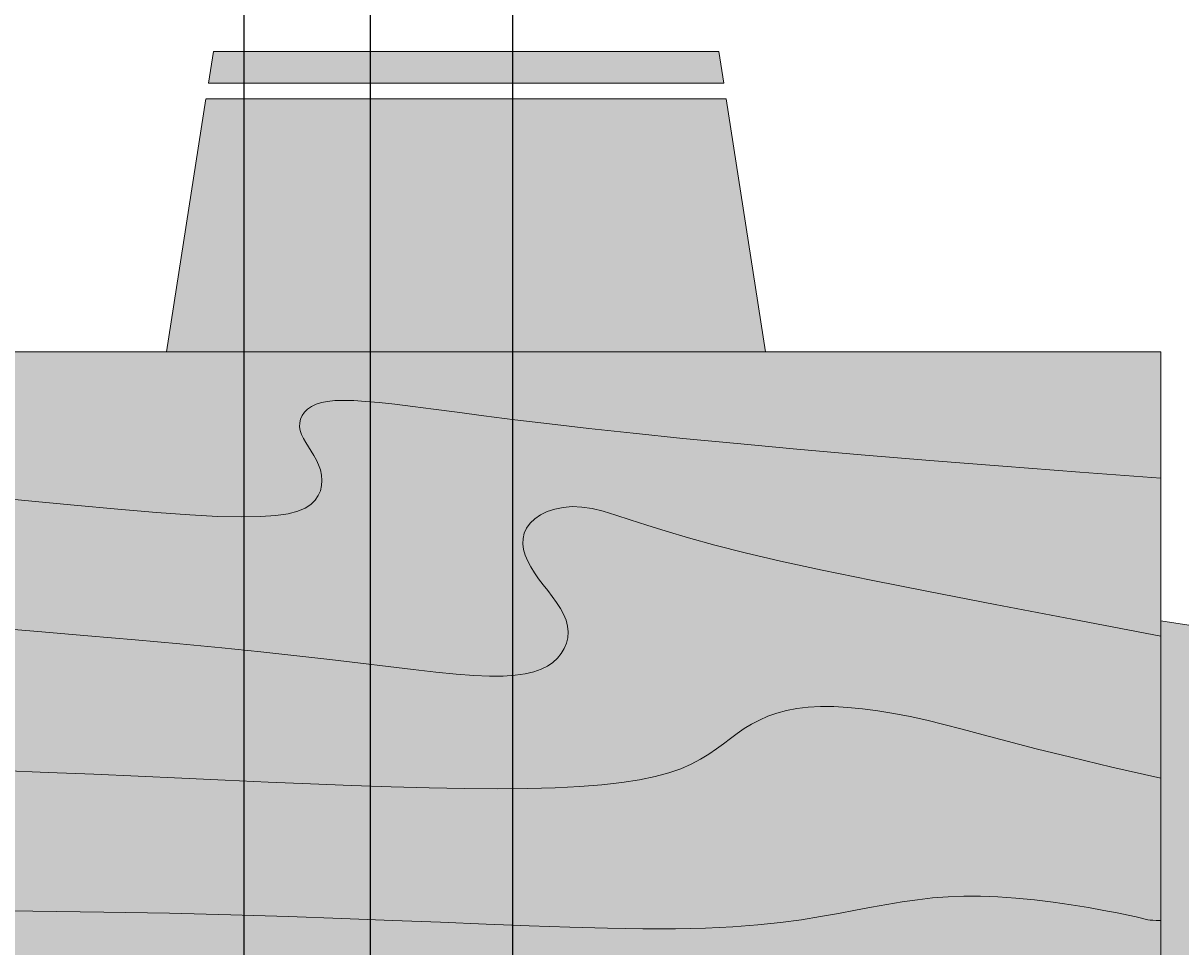
# Model space of a CAD drawing. Units: inches. Extents: x 1567 to 1964, y 1813 to 2447.
# Tile 20 of 28: x 1788 to 1825, y 2199 to 2228. Entities that reach past the tile are written whole.
import ezdxf

# ---------------------------------------------------------------- set-up
doc = ezdxf.new("R2010")
doc.units = ezdxf.units.IN
doc.layers.add('A-ANNO-DIMS', color=2, linetype='Continuous', lineweight=18)
doc.layers.add('A-FURN', color=8, linetype='Continuous', lineweight=18)
doc.layers.add('A-FURN-PATT', color=252, linetype='Continuous', lineweight=13, true_color=0x939598)
doc.styles.get("Standard").update_dxf_attribs({"font": 'arial.ttf'})
doc.dimstyles.get("Standard").update_dxf_attribs({"dimtxt": 0.18, "dimasz": 0.18, "dimexe": 0.18, "dimexo": 0.0625, "dimgap": 0.09, "dimtad": 0, "dimtih": 1, "dimtoh": 1, "dimdec": 4, "dimzin": 0, "dimdsep": 46, "dimtxsty": 'Standard', "dimcen": 0.09, "dimadec": 0, "dimazin": 0, "dimtfac": 1, "dimtdec": 4, "dimtofl": 0, "dimtmove": 0, "dimatfit": 3, "dimfxl": 1, "dimtolj": 1, "dimtzin": 0, "dimarcsym": 0})

# ---------------------------------------------------------------- blocks, each defined once
blk = doc.blocks.new('Dining Set - 36 x 72 in.')
for p, q in [((6, 27.5), (5.8438, 26.50042)), ((6, 27.5), (22, 27.5)), ((22.1563, 26.49966), (22, 27.5)), ((22.1584, 26.5), (5.8466, 26.5)), ((5.7657, 26.00059), (4.5153, 17.99762)), ((5.7696, 26), (22.2392, 26)), ((23.4848, 17.99762), (22.2345, 25.99926)), ((36, 18), (-36, 18)), ((36, -18), (36, 18)), ((44.0006, 8.23428), (35.9976, 9.48474))]:
    blk.add_line(p, q)
for points in [[(-1.6954, 13.45508), (0.0365, 13.29166), (1.5945, 13.14388), (2.9811, 13.01562), (4.1988, 12.9108), (5.25, 12.83333), (6.1393, 12.78613), (6.8802, 12.76823), (7.4883, 12.77767), (7.9792, 12.8125), (8.3685, 12.87077), (8.6719, 12.95052), (8.9049, 13.0498), (9.0833, 13.16666), (9.2205, 13.29899), (9.3216, 13.44401), (9.3895, 13.59879), (9.4271, 13.76041), (9.4373, 13.92594), (9.4232, 14.09245), (9.3875, 14.257), (9.3333, 14.41666), (9.2638, 14.56917), (9.1836, 14.71484), (9.0975, 14.85465), (9.0104, 14.98958), (8.9272, 15.1206), (8.8529, 15.2487), (8.7922, 15.37483), (8.75, 15.5), (8.7305, 15.62467), (8.7344, 15.74739), (8.7617, 15.86621), (8.8125, 15.97916), (8.8867, 16.08431), (8.9844, 16.17968), (9.1055, 16.26334), (9.25, 16.33333), (9.4189, 16.38802), (9.6172, 16.42708), (9.8506, 16.45052), (10.125, 16.45833), (10.4463, 16.45052), (10.8203, 16.42708), (11.2529, 16.38802), (11.75, 16.33333), (12.3184, 16.26318), (12.9694, 16.17838), (13.7151, 16.07991), (14.5677, 15.96875), (15.5395, 15.84586), (16.6426, 15.71224), (17.8893, 15.56884), (19.2917, 15.41666), (20.859, 15.25667), (22.5879, 15.08984), (24.4721, 14.91715), (26.5052, 14.73958), (28.6809, 14.5581), (30.9929, 14.3737), (33.4347, 14.18733), (36, 14)], [(-1.2246, 9.28515), (0.4415, 9.14534), (2.026, 9.01041), (3.5266, 8.87939), (4.9408, 8.7513), (6.266, 8.62516), (7.5, 8.5), (8.6411, 8.37549), (9.6914, 8.2539), (10.6538, 8.13818), (11.5312, 8.03125), (12.3267, 7.93603), (13.043, 7.85547), (13.6831, 7.79248), (14.25, 7.75), (14.7471, 7.7303), (15.1797, 7.73307), (15.5537, 7.75732), (15.875, 7.80208), (16.1494, 7.86637), (16.3828, 7.94922), (16.5811, 8.04964), (16.75, 8.16666), (16.8944, 8.29915), (17.0143, 8.44531), (17.1089, 8.60319), (17.1771, 8.77083), (17.218, 8.94629), (17.2305, 9.1276), (17.2137, 9.31282), (17.1667, 9.5), (17.0895, 9.6875), (16.987, 9.875), (16.8649, 10.0625), (16.7292, 10.25), (16.5856, 10.4375), (16.4401, 10.625), (16.2985, 10.8125), (16.1667, 11), (16.05, 11.18733), (15.9518, 11.3737), (15.8752, 11.5581), (15.8229, 11.73958), (15.798, 11.91715), (15.8034, 12.08984), (15.842, 12.25667), (15.9167, 12.41666), (16.0295, 12.56836), (16.1784, 12.70833), (16.3605, 12.83268), (16.5729, 12.9375), (16.8127, 13.01888), (17.0768, 13.07291), (17.3625, 13.0957), (17.6667, 13.08333), (17.9894, 13.03312), (18.3418, 12.94726), (18.7382, 12.82918), (19.1927, 12.68229), (19.7195, 12.51001), (20.3327, 12.31575), (21.0465, 12.10294), (21.875, 11.875), (22.8357, 11.63354), (23.959, 11.37304), (25.2786, 11.08618), (26.8282, 10.76562), (28.6414, 10.40405), (30.752, 9.99414), (33.1936, 9.52856), (36, 9)], [(-0.7396, 4.73958), (0.7739, 4.6831), (2.22, 4.6237), (3.6213, 4.56233), (5, 4.5), (6.373, 4.43782), (7.7344, 4.3776), (9.0723, 4.32129), (10.375, 4.27083), (11.6309, 4.22819), (12.8281, 4.19531), (13.9551, 4.17415), (15, 4.16666), (15.954, 4.17448), (16.819, 4.19791), (17.6001, 4.23698), (18.3021, 4.29166), (18.9299, 4.36198), (19.4883, 4.44791), (19.9823, 4.54948), (20.4167, 4.66666), (20.7969, 4.79899), (21.1302, 4.94401), (21.4245, 5.09879), (21.6875, 5.26041), (21.9271, 5.42594), (22.1511, 5.59245), (22.3672, 5.757), (22.5834, 5.91666), (22.8065, 6.06868), (23.0404, 6.21093), (23.2879, 6.34147), (23.5521, 6.45833), (23.8358, 6.55957), (24.142, 6.64323), (24.4735, 6.70735), (24.8334, 6.75), (25.2235, 6.76969), (25.642, 6.76692), (26.0858, 6.74267), (26.5521, 6.69791), (27.0379, 6.63362), (27.5404, 6.55078), (28.0565, 6.45036), (28.5834, 6.33333), (29.1242, 6.19987), (29.7071, 6.04687), (30.3661, 5.87044), (31.1354, 5.66666), (32.0493, 5.43164), (33.142, 5.16146), (34.4475, 4.85221), (36, 4.5)], [(-2.134, 0.29793), (0.2878, 0.28711), (2.5317, 0.26163), (4.6146, 0.22396), (6.5529, 0.17651), (8.3633, 0.12174), (10.0623, 0.06209), (11.6667, 0), (13.1899, -0.06201), (14.6341, -0.1211), (15.9982, -0.17432), (17.2813, -0.21875), (18.4823, -0.25147), (19.6003, -0.26953), (20.6343, -0.27002), (21.5834, -0.25), (22.4481, -0.20768), (23.2357, -0.14584), (23.9549, -0.06836), (24.6146, 0.02083), (25.2235, 0.11784), (25.7904, 0.21875), (26.3241, 0.31966), (26.8334, 0.41666), (27.3265, 0.50618), (27.8099, 0.58593), (28.2894, 0.65397), (28.7709, 0.70833), (29.2601, 0.74707), (29.763, 0.76823), (30.2855, 0.76985), (30.8334, 0.75), (31.4088, 0.70784), (31.9994, 0.64713), (32.589, 0.57275), (33.1615, 0.48958), (33.7008, 0.4025), (34.1908, 0.3164), (34.6153, 0.23616), (34.9584, 0.16666), (35.2099, 0.11165), (35.3848, 0.07031), (35.504, 0.04069), (35.5886, 0.02083), (35.6594, 0.00879), (35.7377, 0.0026), (35.8442, 0.00032), (36, 0)]]:
    blk.add_lwpolyline(points)
blk = doc.blocks.new('*D54')
at = {"layer": 'A-ANNO-DIMS', "color": 0, "lineweight": -2, "transparency": 16777216}
for p, q in [((1711.43, 1964.352), (1711.43, 2447.12)), ((1711.61, 2446.94), (1753.211, 2446.94)), ((1795.25, 2446.94), (1753.648, 2446.94)), ((1795.43, 1964.352), (1795.43, 2447.12))]:
    blk.add_line(p, q, dxfattribs=at)
at = {"layer": 'A-ANNO-DIMS', "color": 0, "transparency": 16777216}
for points in [[(1711.61, 2446.97), (1711.61, 2446.91), (1711.43, 2446.94)], [(1795.25, 2446.97), (1795.25, 2446.91), (1795.43, 2446.94)]]:
    blk.add_solid(points, dxfattribs=at)
at = {"layer": 'Defpoints', "color": 0, "transparency": 16777216}
for p in [(1795.43, 2446.94), (1711.43, 1964.29), (1795.43, 1964.29)]:
    blk.add_point(p, dxfattribs=at)
at = {"layer": 'A-ANNO-DIMS', "color": 0, "transparency": 16777216, "insert": (1753.43, 2446.94), "char_height": 0.18, "attachment_point": 5}
blk.add_mtext('\\A1;84', dxfattribs=at)
blk = doc.blocks.new('*D55')
at = {"layer": 'A-ANNO-DIMS', "color": 0, "lineweight": -2, "transparency": 16777216}
for p, q in [((1795.43, 1964.352), (1795.43, 2447.12)), ((1795.61, 2446.94), (1797.277, 2446.94)), ((1799.25, 2446.94), (1797.582, 2446.94)), ((1799.43, 1967.352), (1799.43, 2447.12))]:
    blk.add_line(p, q, dxfattribs=at)
at = {"layer": 'A-ANNO-DIMS', "color": 0, "transparency": 16777216}
for points in [[(1795.61, 2446.97), (1795.61, 2446.91), (1795.43, 2446.94)], [(1799.25, 2446.97), (1799.25, 2446.91), (1799.43, 2446.94)]]:
    blk.add_solid(points, dxfattribs=at)
at = {"layer": 'Defpoints', "color": 0, "transparency": 16777216}
for p in [(1799.43, 2446.94), (1799.43, 1967.29), (1795.43, 1964.29)]:
    blk.add_point(p, dxfattribs=at)
at = {"layer": 'A-ANNO-DIMS', "color": 0, "transparency": 16777216, "insert": (1797.43, 2446.94), "char_height": 0.18, "attachment_point": 5}
blk.add_mtext('\\A1;4', dxfattribs=at)
blk = doc.blocks.new('*D70')
at = {"layer": 'A-ANNO-DIMS', "color": 0, "lineweight": -2, "transparency": 16777216}
for p, q in [((1799.43, 1967.352), (1799.43, 2447.12)), ((1799.61, 2446.94), (1801.421, 2446.94)), ((1803.75, 2446.94), (1801.938, 2446.94)), ((1803.93, 1967.352), (1803.93, 2447.12))]:
    blk.add_line(p, q, dxfattribs=at)
at = {"layer": 'A-ANNO-DIMS', "color": 0, "transparency": 16777216}
for points in [[(1799.61, 2446.97), (1799.61, 2446.91), (1799.43, 2446.94)], [(1803.75, 2446.97), (1803.75, 2446.91), (1803.93, 2446.94)]]:
    blk.add_solid(points, dxfattribs=at)
at = {"layer": 'Defpoints', "color": 0, "transparency": 16777216}
for p in [(1803.93, 2446.94), (1799.43, 1967.29), (1803.93, 1967.29)]:
    blk.add_point(p, dxfattribs=at)
at = {"layer": 'A-ANNO-DIMS', "color": 0, "transparency": 16777216, "insert": (1801.68, 2446.94), "char_height": 0.18, "attachment_point": 5}
blk.add_mtext('\\A1;4.5', dxfattribs=at)
blk = doc.blocks.new('*D71')
at = {"layer": 'A-ANNO-DIMS', "color": 0, "lineweight": -2, "transparency": 16777216}
for p, q in [((1799.43, 1910.752), (1799.43, 2447.12)), ((1799.61, 2446.94), (1861.648, 2446.94)), ((1924.25, 2446.94), (1862.211, 2446.94)), ((1924.43, 1910.752), (1924.43, 2447.12))]:
    blk.add_line(p, q, dxfattribs=at)
at = {"layer": 'A-ANNO-DIMS', "color": 0, "transparency": 16777216}
for points in [[(1799.61, 2446.97), (1799.61, 2446.91), (1799.43, 2446.94)], [(1924.25, 2446.97), (1924.25, 2446.91), (1924.43, 2446.94)]]:
    blk.add_solid(points, dxfattribs=at)
at = {"layer": 'Defpoints', "color": 0, "transparency": 16777216}
for p in [(1924.43, 2446.94), (1799.43, 1910.69), (1924.43, 1910.69)]:
    blk.add_point(p, dxfattribs=at)
at = {"layer": 'A-ANNO-DIMS', "color": 0, "transparency": 16777216, "insert": (1861.93, 2446.94), "char_height": 0.18, "attachment_point": 5}
blk.add_mtext('\\A1;125', dxfattribs=at)

msp = doc.modelspace()

# ---------------------------------------------------------------- hatches: boundary and pattern name
at = {"layer": 'A-FURN-PATT'}
h = msp.add_hatch(color=256, dxfattribs=at)
h.dxf.hatch_style = 1
h.paths.add_polyline_path([(1621.2532, 2242.0229), (1643.7811, 2241.7239), (1643.8607, 2247.7234), (1617.863, 2248.0685, 0.1904762), (1616.7481, 2164.0759), (1642.7458, 2163.7308), (1642.8254, 2169.7302), (1620.2975, 2170.0293, -0.1519478)])
h.paths.add_polyline_path([(1673.5306, 2249.6607), (1653.8509, 2249.6607), (1653.8509, 2248.5031, 0.1176471), (1673.5306, 2248.5031)])
h.paths.add_polyline_path([(1706.0889, 2249.6607), (1686.4092, 2249.6607), (1686.4092, 2248.5031, 0.1176471), (1706.0889, 2248.5031)])
h.paths.add_polyline_path([(1782.4511, 2227.4197), (1766.4511, 2227.4197), (1766.2949, 2226.4197), (1782.6074, 2226.4197)])
h.paths.add_polyline_path([(1810.4511, 2227.4197), (1794.4511, 2227.4197), (1794.2949, 2226.4197), (1810.6074, 2226.4197)])
h.paths.add_polyline_path([(1743.9511, 2208.076), (1742.9511, 2207.9197), (1742.9511, 2191.9197), (1743.9511, 2191.7635)])
h.paths.add_polyline_path([(1782.6074, 2173.4197), (1766.2949, 2173.4197), (1766.4511, 2172.4197), (1782.4511, 2172.4197)])
h.paths.add_polyline_path([(1810.6074, 2173.4197), (1794.2949, 2173.4197), (1794.4511, 2172.4197), (1810.4511, 2172.4197)])
h.paths.add_polyline_path([(1861.053, 2006.5071), (1845.8531, 2006.5071), (1861.053, 1991.3071)])
h.paths.add_polyline_path([(1905.853, 1993.7071), (1861.053, 1993.7071), (1861.053, 1991.3071), (1905.853, 1991.3071)])
h.paths.add_polyline_path([(1919.7245, 2257.29, 0.5000001), (1918.7245, 2258.29), (1901.7245, 2258.29, 0.5000001), (1900.7245, 2257.29), (1900.7245, 2253.29, 0.5000001), (1901.7245, 2252.29), (1918.7245, 2252.29, 0.5000001), (1919.7245, 2253.29)])
h.paths.add_polyline_path([(1875.9094, 2391.0204), (1875.9094, 2375.8204), (1891.1093, 2375.8204)], flags=17)
h.paths.add_polyline_path([(1891.1093, 2405.4204), (1831.1094, 2405.4204), (1831.1094, 2391.0204), (1839.1093, 2391.0204), (1839.1093, 2404.2204), (1859.9093, 2404.2204), (1859.9093, 2391.0204), (1862.3093, 2391.0204), (1862.3093, 2404.2204), (1883.1093, 2404.2204), (1883.1093, 2389.0204), (1877.9094, 2389.0204), (1891.1093, 2375.8204)])
h.paths.add_polyline_path([(1682.1402, 2390.0316), (1682.1402, 2374.8316), (1697.3402, 2374.8316)], flags=17)
h.paths.add_polyline_path([(1697.3402, 2404.4316), (1637.3402, 2404.4316), (1637.3402, 2390.0316), (1645.3402, 2390.0316), (1645.3402, 2403.2316), (1666.1402, 2403.2316), (1666.1402, 2390.0316), (1668.5402, 2390.0316), (1668.5402, 2403.2316), (1689.3402, 2403.2316), (1689.3402, 2388.0316), (1684.1402, 2388.0316), (1697.3402, 2374.8316)])
h = msp.add_hatch(color=256, dxfattribs=at)
h.dxf.hatch_style = 1
h.paths.add_polyline_path([(1697.3402, 2374.8316), (1682.1402, 2374.8316), (1682.1402, 2387.6316), (1637.3402, 2387.6316), (1637.3402, 2324.4315), (1697.3402, 2324.4315)])
h.paths.add_polyline_path([(1891.1093, 2375.8204), (1875.9094, 2375.8204), (1875.9094, 2388.6204), (1831.1094, 2388.6204), (1831.1094, 2325.4204), (1891.1093, 2325.4204)])
h.paths.add_polyline_path([(1702.5611, 2206.8057), (1702.5611, 2210.8057), (1699.7395, 2209.9436), (1697.013, 2209.2403), (1694.3857, 2208.6763), (1691.8615, 2208.2326), (1689.4443, 2207.8896), (1687.1381, 2207.6282), (1684.9469, 2207.4289), (1682.8747, 2207.2725), (1680.9233, 2207.1425), (1679.0865, 2207.0339), (1677.3558, 2206.9445), (1675.7229, 2206.8719), (1674.1794, 2206.8141), (1672.7169, 2206.7688), (1671.327, 2206.7339), (1670.0014, 2206.707), (1668.7314, 2206.6866), (1667.5072, 2206.6732), (1666.3188, 2206.668), (1665.1561, 2206.6722), (1664.009, 2206.6869), (1662.8675, 2206.7133), (1661.7215, 2206.7525), (1660.5611, 2206.8057), (1660.5611, 2202.8057), (1661.9932, 2202.9556), (1663.3314, 2203.0744), (1664.5899, 2203.1671), (1665.7831, 2203.2385), (1666.9254, 2203.2935), (1668.0311, 2203.3368), (1669.1145, 2203.3734), (1670.1902, 2203.4081), (1671.2724, 2203.4451), (1672.3759, 2203.4866), (1673.5155, 2203.534), (1674.706, 2203.5887), (1675.9621, 2203.6523), (1677.2986, 2203.7262), (1678.7304, 2203.8118), (1680.2722, 2203.9108), (1681.947, 2204.0272), (1683.8108, 2204.1769), (1685.9279, 2204.3782), (1688.3626, 2204.6496), (1691.179, 2205.0096), (1694.4413, 2205.4767), (1698.214, 2206.0692)])
h.paths.add_polyline_path([(1702.5611, 2218.8057), (1701.9821, 2217.9383), (1701.3316, 2217.191), (1700.6091, 2216.5515), (1699.8141, 2216.0071), (1698.946, 2215.5454), (1698.0041, 2215.1536), (1696.9879, 2214.8194), (1695.8969, 2214.5301), (1694.7328, 2214.2753), (1693.5072, 2214.0522), (1692.2339, 2213.8602), (1690.9266, 2213.6989), (1689.5994, 2213.5675), (1688.266, 2213.4654), (1686.9402, 2213.392), (1685.636, 2213.3467), (1684.3619, 2213.3287), (1683.1053, 2213.3361), (1681.8482, 2213.3668), (1680.5727, 2213.4187), (1679.2608, 2213.4898), (1677.8948, 2213.5779), (1676.4565, 2213.6811), (1674.9282, 2213.7971), (1673.2982, 2213.9236), (1671.5804, 2214.0573), (1669.795, 2214.1945), (1667.9622, 2214.3316), (1666.1022, 2214.4649), (1664.2352, 2214.5908), (1662.3814, 2214.7056), (1660.5611, 2214.8057), (1660.5611, 2206.8057), (1661.7215, 2206.7525), (1662.8675, 2206.7133), (1664.009, 2206.6869), (1665.1561, 2206.6722), (1666.3188, 2206.668), (1667.5072, 2206.6732), (1668.7314, 2206.6866), (1670.0014, 2206.707), (1671.327, 2206.7339), (1672.7169, 2206.7688), (1674.1794, 2206.8141), (1675.7229, 2206.8719), (1677.3558, 2206.9445), (1679.0865, 2207.0339), (1680.9233, 2207.1425), (1682.8747, 2207.2725), (1684.9469, 2207.4289), (1687.1381, 2207.6282), (1689.4443, 2207.8896), (1691.8615, 2208.2326), (1694.3857, 2208.6763), (1697.013, 2209.2403), (1699.7395, 2209.9436), (1702.5611, 2210.8057)])
h.paths.add_polyline_path([(1700.6091, 2216.5515), (1701.3316, 2217.191), (1701.9821, 2217.9383), (1702.5611, 2218.8057), (1702.5611, 2222.8057), (1689.452, 2222.8057), (1689.0171, 2222.4556), (1688.4521, 2222.0354), (1687.7806, 2221.5662), (1687.0235, 2221.067), (1686.2019, 2220.5566), (1685.3367, 2220.0541), (1684.4491, 2219.5785), (1683.56, 2219.1486), (1682.6867, 2218.7795), (1681.8312, 2218.4692), (1680.9918, 2218.212), (1680.1667, 2218.0019), (1679.3541, 2217.833), (1678.5524, 2217.6995), (1677.7597, 2217.5954), (1676.9744, 2217.5149), (1676.1942, 2217.4531), (1675.4146, 2217.4093), (1674.6309, 2217.384), (1673.8381, 2217.3774), (1673.0313, 2217.39), (1672.2056, 2217.4221), (1671.3562, 2217.4741), (1670.4782, 2217.5463), (1669.5642, 2217.639), (1668.5968, 2217.7516), (1667.5562, 2217.8833), (1666.4226, 2218.0336), (1665.1761, 2218.2017), (1663.7969, 2218.3869), (1662.2651, 2218.5885), (1660.5611, 2218.8057), (1660.5611, 2214.8057), (1662.3814, 2214.7056), (1664.2352, 2214.5908), (1666.1022, 2214.4649), (1667.9622, 2214.3316), (1669.795, 2214.1945), (1671.5804, 2214.0573), (1673.2982, 2213.9236), (1674.9282, 2213.7971), (1676.4565, 2213.6811), (1677.8948, 2213.5779), (1679.2608, 2213.4898), (1680.5727, 2213.4187), (1681.8482, 2213.3668), (1683.1053, 2213.3361), (1684.3619, 2213.3287), (1685.636, 2213.3467), (1686.9402, 2213.392), (1688.266, 2213.4654), (1689.5994, 2213.5675), (1690.9266, 2213.6989), (1692.2339, 2213.8602), (1693.5072, 2214.0522), (1694.7328, 2214.2753), (1695.8969, 2214.5301), (1696.9879, 2214.8194), (1698.0041, 2215.1536), (1698.946, 2215.5454), (1699.8141, 2216.0071)])
h.paths.add_polyline_path([(1687.0235, 2221.067), (1687.7806, 2221.5662), (1688.4521, 2222.0354), (1689.0171, 2222.4556), (1689.452, 2222.8057), (1660.5611, 2222.8057), (1660.5611, 2218.8057), (1662.2651, 2218.5885), (1663.7969, 2218.3869), (1665.1761, 2218.2017), (1666.4226, 2218.0336), (1667.5562, 2217.8833), (1668.5968, 2217.7516), (1669.5642, 2217.639), (1670.4782, 2217.5463), (1671.3562, 2217.4741), (1672.2056, 2217.4221), (1673.0313, 2217.39), (1673.8381, 2217.3774), (1674.6309, 2217.384), (1675.4146, 2217.4093), (1676.1942, 2217.4531), (1676.9744, 2217.5149), (1677.7597, 2217.5954), (1678.5524, 2217.6995), (1679.3541, 2217.833), (1680.1667, 2218.0019), (1680.9918, 2218.212), (1681.8312, 2218.4692), (1682.6867, 2218.7795), (1683.56, 2219.1486), (1684.4491, 2219.5785), (1685.3367, 2220.0541), (1686.2019, 2220.5566)], flags=17)
h.paths.add_polyline_path([(1702.5611, 2198.8057), (1698.9289, 2199.2412), (1695.8472, 2199.5774), (1693.2166, 2199.8257), (1690.9377, 2199.9973), (1688.9111, 2200.1033), (1687.0375, 2200.155), (1685.2174, 2200.1637), (1683.3514, 2200.1406), (1681.3514, 2200.0941), (1679.1736, 2200.0225), (1676.7858, 2199.921), (1674.1554, 2199.7852), (1671.2502, 2199.6103), (1668.0377, 2199.3919), (1664.4854, 2199.1252), (1660.5611, 2198.8057), (1660.5611, 2194.8057), (1662.2697, 2194.9771), (1663.9673, 2195.0999), (1665.6339, 2195.1809), (1667.2495, 2195.227), (1668.7941, 2195.2449), (1670.2478, 2195.2414), (1671.5906, 2195.2233), (1672.8026, 2195.1974), (1673.8739, 2195.1689), (1674.8359, 2195.1364), (1675.7302, 2195.0967), (1676.5982, 2195.0469), (1677.4817, 2194.9838), (1678.422, 2194.9043), (1679.4609, 2194.8055), (1680.6397, 2194.6842), (1682.005, 2194.5341), (1683.6223, 2194.335), (1685.562, 2194.0637), (1687.8945, 2193.6967), (1690.6902, 2193.2108), (1694.0196, 2192.5826), (1697.9531, 2191.7887), (1702.5611, 2190.8057)])
h.paths.add_polyline_path([(1702.5611, 2206.8057), (1698.214, 2206.0692), (1694.4413, 2205.4767), (1691.179, 2205.0096), (1688.3626, 2204.6496), (1685.9279, 2204.3782), (1683.8108, 2204.1769), (1681.947, 2204.0272), (1680.2722, 2203.9108), (1678.7304, 2203.8118), (1677.2986, 2203.7262), (1675.9621, 2203.6523), (1674.706, 2203.5887), (1673.5155, 2203.534), (1672.3759, 2203.4866), (1671.2724, 2203.4451), (1670.1902, 2203.4081), (1669.1145, 2203.3734), (1668.0311, 2203.3368), (1666.9254, 2203.2935), (1665.7831, 2203.2385), (1664.5899, 2203.1671), (1663.3314, 2203.0744), (1661.9932, 2202.9556), (1660.5611, 2202.8057), (1660.5611, 2198.8057), (1664.4854, 2199.1252), (1668.0377, 2199.3919), (1671.2502, 2199.6103), (1674.1554, 2199.7852), (1676.7858, 2199.921), (1679.1736, 2200.0225), (1681.3514, 2200.0941), (1683.3514, 2200.1406), (1685.2174, 2200.1637), (1687.0375, 2200.155), (1688.9111, 2200.1033), (1690.9377, 2199.9973), (1693.2166, 2199.8257), (1695.8472, 2199.5774), (1698.9289, 2199.2412), (1702.5611, 2198.8057)])
h.paths.add_polyline_path([(1702.5611, 2190.8057), (1697.9531, 2191.7887), (1694.0196, 2192.5826), (1690.6902, 2193.2108), (1687.8945, 2193.6967), (1685.562, 2194.0637), (1683.6223, 2194.335), (1682.005, 2194.5341), (1680.6397, 2194.6842), (1679.4609, 2194.8055), (1678.422, 2194.9043), (1677.4817, 2194.9838), (1676.5982, 2195.0469), (1675.7302, 2195.0967), (1674.8359, 2195.1364), (1673.8739, 2195.1689), (1672.8026, 2195.1974), (1671.5906, 2195.2233), (1670.2478, 2195.2414), (1668.7941, 2195.2449), (1667.2495, 2195.227), (1665.6339, 2195.1809), (1663.9673, 2195.0999), (1662.2697, 2194.9771), (1660.5611, 2194.8057), (1660.5611, 2190.8057), (1665.9637, 2190.2699), (1670.5105, 2189.7867), (1674.3035, 2189.3504), (1677.4445, 2188.9552), (1680.0354, 2188.5951), (1682.1782, 2188.2644), (1683.9747, 2187.9571), (1685.5268, 2187.6675), (1686.9225, 2187.3901), (1688.1943, 2187.1216), (1689.3606, 2186.859), (1690.4399, 2186.5993), (1691.4508, 2186.3396), (1692.4118, 2186.0769), (1693.3413, 2185.8084), (1694.2579, 2185.531), (1695.1786, 2185.2422), (1696.1142, 2184.9406), (1697.0739, 2184.6252), (1698.0671, 2184.2949), (1699.1032, 2183.9489), (1700.1913, 2183.586), (1701.3408, 2183.2053), (1702.5611, 2182.8057)])
h.paths.add_polyline_path([(1702.5611, 2182.8057), (1701.3408, 2183.2053), (1700.1913, 2183.586), (1699.1032, 2183.9489), (1698.0671, 2184.2949), (1697.0739, 2184.6252), (1696.1142, 2184.9406), (1695.1786, 2185.2422), (1694.2579, 2185.531), (1693.3413, 2185.8084), (1692.4118, 2186.0769), (1691.4508, 2186.3396), (1690.4399, 2186.5993), (1689.3606, 2186.859), (1688.1943, 2187.1216), (1686.9225, 2187.3901), (1685.5268, 2187.6675), (1683.9747, 2187.9571), (1682.1782, 2188.2644), (1680.0354, 2188.5951), (1677.4445, 2188.9552), (1674.3035, 2189.3504), (1670.5105, 2189.7867), (1665.9637, 2190.2699), (1660.5611, 2190.8057), (1660.5611, 2186.8057), (1663.5709, 2186.52), (1666.0965, 2186.2414), (1668.1979, 2185.9698), (1669.9351, 2185.7048), (1671.3681, 2185.446), (1672.5568, 2185.1931), (1673.5613, 2184.9458), (1674.4415, 2184.7037), (1675.2485, 2184.4664), (1675.9976, 2184.2328), (1677.0295, 2183.8907), (1678.2492, 2183.4332), (1679.354, 2182.9669), (1680.4123, 2182.4724), (1681.3757, 2181.9718), (1682.2435, 2181.4594), (1683.1864, 2180.8057), (1702.5611, 2180.8057)])
h.paths.add_polyline_path([(1677.3469, 2183.7716), (1676.6949, 2184.0016), (1675.9976, 2184.2328), (1675.2485, 2184.4664), (1674.4415, 2184.7037), (1673.5613, 2184.9458), (1672.5568, 2185.1931), (1671.3681, 2185.446), (1669.9351, 2185.7048), (1668.1979, 2185.9698), (1666.0965, 2186.2414), (1663.5709, 2186.52), (1660.5611, 2186.8057), (1660.5611, 2180.8057), (1683.1506, 2180.8057), (1682.802, 2181.0722), (1682.4264, 2181.3326), (1682.0201, 2181.5913), (1681.586, 2181.8476), (1681.1268, 2182.1011), (1680.6453, 2182.3513), (1680.1443, 2182.5976), (1679.6266, 2182.8395), (1679.0933, 2183.0769), (1678.5398, 2183.3105), (1677.9598, 2183.5417)], flags=17)
h.paths.add_polyline_path([(1824.4511, 2199.9016), (1824.089, 2199.9302), (1824.0595, 2199.9372), (1824.0397, 2199.9406), (1823.5413, 2200.0576), (1823.4095, 2200.0864), (1823.0664, 2200.1559), (1822.6419, 2200.2361), (1822.1519, 2200.3222), (1821.6126, 2200.4093), (1821.0401, 2200.4925), (1820.4505, 2200.5669), (1819.8599, 2200.6276), (1819.2845, 2200.6697), (1818.7366, 2200.6896), (1818.2141, 2200.688), (1817.7112, 2200.6668), (1817.222, 2200.6281), (1816.7405, 2200.5737), (1816.261, 2200.5057), (1815.7776, 2200.4259), (1815.2845, 2200.3364), (1814.3007, 2200.149), (1813.3315, 2199.9765), (1812.406, 2199.8514), (1811.6868, 2199.7739), (1810.8992, 2199.7121), (1810.0345, 2199.6697), (1809.0854, 2199.6497), (1808.0514, 2199.6502), (1806.9334, 2199.6683), (1805.7324, 2199.701), (1804.4493, 2199.7454), (1803.0852, 2199.7986), (1801.641, 2199.8577), (1800.1178, 2199.9197), (1798.5134, 2199.9818), (1796.8144, 2200.0415), (1795.004, 2200.0962), (1793.0657, 2200.1437), (1790.9828, 2200.1814), (1788.7389, 2200.2068), (1786.3171, 2200.2177), (1783.7011, 2200.2114), (1780.8715, 2200.185), (1777.7988, 2200.1326), (1774.4506, 2200.0481), (1770.7948, 2199.9249), (1766.7992, 2199.7569), (1762.4316, 2199.5376), (1757.6596, 2199.2606), (1752.4511, 2198.9197), (1752.4511, 2193.4197), (1761.2668, 2193.6071), (1768.3671, 2193.7934), (1773.9821, 2193.9778), (1778.3417, 2194.1593), (1781.6759, 2194.3369), (1784.2148, 2194.5096), (1786.1882, 2194.6764), (1787.8261, 2194.8364), (1789.3219, 2194.9887), (1790.7226, 2195.1333), (1792.0383, 2195.27), (1793.2792, 2195.3989), (1794.4557, 2195.52), (1795.5781, 2195.6333), (1796.6564, 2195.7387), (1797.7011, 2195.8364), (1798.7216, 2195.9259), (1799.7245, 2196.0057), (1800.7158, 2196.0737), (1801.7011, 2196.1281), (1802.6865, 2196.1668), (1803.6777, 2196.188), (1804.6806, 2196.1896), (1805.7011, 2196.1697), (1806.7423, 2196.1273), (1807.7962, 2196.0643), (1808.852, 2195.9837), (1809.899, 2195.8885), (1810.9265, 2195.7815), (1811.9238, 2195.6658), (1812.88, 2195.5442), (1813.7845, 2195.4197), (1814.6296, 2195.2948), (1815.4205, 2195.1704), (1816.1656, 2195.0469), (1816.873, 2194.9249), (1817.5511, 2194.8049), (1818.2083, 2194.6873), (1818.8527, 2194.5726), (1819.4928, 2194.4614), (1820.1348, 2194.3554), (1820.7773, 2194.2615), (1821.4169, 2194.1882), (1822.0501, 2194.1437), (1822.6735, 2194.1363), (1823.2838, 2194.1743), (1823.8775, 2194.266), (1824.4511, 2194.4197)])
h.paths.add_polyline_path([(1821.4716, 2190.5098), (1820.4303, 2190.5708), (1819.3811, 2190.6415), (1818.3339, 2190.7186), (1817.2985, 2190.7986), (1816.2845, 2190.8781), (1815.2976, 2190.9542), (1814.3274, 2191.0259), (1813.3592, 2191.0927), (1812.3782, 2191.1541), (1811.3699, 2191.2097), (1810.3196, 2191.2589), (1809.2127, 2191.3013), (1808.0345, 2191.3364), (1806.7708, 2191.3634), (1805.4094, 2191.3807), (1803.9387, 2191.3862), (1802.3469, 2191.3781), (1800.6223, 2191.3543), (1798.7532, 2191.313), (1796.7278, 2191.2521), (1794.5344, 2191.1697), (1792.128, 2191.0648), (1789.33, 2190.9393), (1785.9285, 2190.7962), (1781.7115, 2190.6385), (1776.4672, 2190.469), (1769.9836, 2190.2908), (1762.0489, 2190.1067), (1752.4511, 2189.9197), (1752.4511, 2185.4197), (1758.363, 2185.5846), (1763.4179, 2185.7075), (1767.7199, 2185.7933), (1771.373, 2185.8468), (1774.4811, 2185.873), (1777.1484, 2185.8768), (1779.4787, 2185.8629), (1781.5761, 2185.8364), (1783.5287, 2185.8014), (1785.3606, 2185.7596), (1787.0802, 2185.7119), (1788.6959, 2185.6593), (1790.2158, 2185.6028), (1791.6484, 2185.5434), (1793.0018, 2185.4821), (1794.2844, 2185.4197), (1795.5065, 2185.3576), (1796.6861, 2185.298), (1797.8433, 2185.2432), (1798.998, 2185.1958), (1800.1703, 2185.1581), (1801.3801, 2185.1326), (1802.6476, 2185.1218), (1803.9928, 2185.1281), (1805.4444, 2185.1555), (1807.0663, 2185.2147), (1808.9315, 2185.3178), (1811.1126, 2185.477), (1813.6823, 2185.7046), (1816.7135, 2186.0128), (1820.2788, 2186.4138), (1824.4511, 2186.9197), (1824.4511, 2190.4197), (1823.4918, 2190.4309), (1822.4954, 2190.4621)])
h.paths.add_polyline_path([(1797.3762, 2216.0584), (1797.6199, 2216.2267), (1797.9558, 2216.3355), (1798.3017, 2216.3703), (1798.5761, 2216.3781), (1798.8974, 2216.3703), (1799.2714, 2216.3468), (1799.704, 2216.3078), (1800.2011, 2216.2531), (1800.7695, 2216.1829), (1801.4205, 2216.0981), (1802.1662, 2215.9996), (1803.0188, 2215.8885), (1803.9906, 2215.7656), (1805.0937, 2215.632), (1806.3404, 2215.4886), (1807.7428, 2215.3364), (1809.3101, 2215.1764), (1811.039, 2215.0096), (1812.9232, 2214.8369), (1814.9563, 2214.6593), (1817.132, 2214.4778), (1819.444, 2214.2934), (1821.8858, 2214.1071), (1824.4511, 2213.9197), (1824.4511, 2217.9197), (1752.4511, 2217.9197), (1752.4511, 2214.9197), (1757.2739, 2214.8973), (1761.6432, 2214.8338), (1765.5973, 2214.7352), (1769.1751, 2214.6072), (1772.4149, 2214.4559), (1775.3554, 2214.2869), (1778.0352, 2214.1063), (1780.4928, 2213.9197), (1782.7607, 2213.7329), (1784.8476, 2213.5499), (1786.7557, 2213.3748), (1788.4876, 2213.2114), (1790.0456, 2213.0636), (1791.4322, 2212.9354), (1792.6499, 2212.8305), (1793.7011, 2212.7531), (1794.5904, 2212.7059), (1795.3313, 2212.688), (1795.9394, 2212.6974), (1796.4303, 2212.7322), (1796.8196, 2212.7905), (1797.123, 2212.8703), (1797.356, 2212.9695), (1797.5344, 2213.0864), (1797.6716, 2213.2187), (1797.7727, 2213.3637), (1797.8406, 2213.5185), (1797.8782, 2213.6801), (1797.8884, 2213.8457), (1797.8743, 2214.0122), (1797.8386, 2214.1767), (1797.7844, 2214.3364), (1797.7149, 2214.4889), (1797.6347, 2214.6346), (1797.5486, 2214.7744), (1797.3327, 2215.109), (1797.178, 2215.4303), (1797.1896, 2215.7939)])
h.paths.add_polyline_path([(1804.7872, 2210.6789), (1804.546, 2211.022), (1804.3512, 2211.3917), (1804.2466, 2211.7546), (1804.2574, 2212.0998), (1804.4058, 2212.4178), (1804.7068, 2212.7007), (1805.1359, 2212.9124), (1805.5279, 2212.9926), (1805.8136, 2213.0154), (1806.1178, 2213.0031), (1806.4405, 2212.9529), (1806.7929, 2212.867), (1807.1893, 2212.7489), (1807.6438, 2212.602), (1808.1706, 2212.4297), (1808.7838, 2212.2355), (1809.4976, 2212.0227), (1810.3261, 2211.7947), (1811.2868, 2211.5533), (1812.4101, 2211.2928), (1813.7297, 2211.0059), (1815.2793, 2210.6854), (1817.0925, 2210.3238), (1819.2031, 2209.9139), (1821.6447, 2209.4483), (1824.4511, 2208.9197), (1824.4511, 2213.9197), (1821.8858, 2214.1071), (1819.444, 2214.2934), (1817.132, 2214.4778), (1814.9563, 2214.6593), (1812.9232, 2214.8369), (1811.039, 2215.0096), (1809.3101, 2215.1764), (1807.7428, 2215.3364), (1806.3404, 2215.4886), (1805.0937, 2215.632), (1803.9906, 2215.7656), (1803.0188, 2215.8885), (1802.1662, 2215.9996), (1801.4205, 2216.0981), (1800.7695, 2216.1829), (1800.2011, 2216.2531), (1799.704, 2216.3078), (1799.2714, 2216.3468), (1798.8974, 2216.3703), (1798.5761, 2216.3781), (1798.3017, 2216.3703), (1798.0683, 2216.3468), (1797.87, 2216.3078), (1797.7011, 2216.2531), (1797.5566, 2216.1831), (1797.4355, 2216.0994), (1797.3378, 2216.004), (1797.2636, 2215.8989), (1797.2128, 2215.7859), (1797.1855, 2215.6671), (1797.1816, 2215.5444), (1797.2011, 2215.4197), (1797.2433, 2215.2946), (1797.304, 2215.1684), (1797.3783, 2215.0403), (1797.4615, 2214.9093), (1797.6718, 2214.5836), (1797.8218, 2214.2545), (1797.8933, 2213.9247), (1797.8728, 2213.5918), (1797.7366, 2213.2814), (1797.4586, 2213.0132), (1797.123, 2212.8703), (1796.8196, 2212.7905), (1796.4303, 2212.7322), (1795.9394, 2212.6974), (1795.3313, 2212.688), (1794.5904, 2212.7059), (1793.7011, 2212.7531), (1792.6499, 2212.8305), (1791.4322, 2212.9354), (1790.0456, 2213.0636), (1788.4876, 2213.2114), (1786.7557, 2213.3748), (1784.8476, 2213.5499), (1782.7607, 2213.7329), (1780.4928, 2213.9197), (1778.0352, 2214.1063), (1775.3554, 2214.2869), (1772.4149, 2214.4559), (1769.1751, 2214.6072), (1765.5973, 2214.7352), (1761.6432, 2214.8338), (1757.2739, 2214.8973), (1752.4511, 2214.9197), (1752.4511, 2209.9197), (1759.4745, 2210.0625), (1765.2786, 2210.1242), (1770.027, 2210.1175), (1773.8834, 2210.0551), (1777.0112, 2209.9498), (1779.5741, 2209.8143), (1781.7357, 2209.6611), (1783.6594, 2209.5031), (1785.4813, 2209.3506), (1787.2265, 2209.2049), (1788.8926, 2209.0651), (1790.4771, 2208.9301), (1791.9777, 2208.7991), (1793.3919, 2208.671), (1794.7171, 2208.5449), (1795.9511, 2208.4197), (1797.0922, 2208.2952), (1798.1425, 2208.1736), (1799.1049, 2208.0579), (1799.9823, 2207.951), (1800.7778, 2207.8558), (1801.4941, 2207.7752), (1802.1342, 2207.7122), (1802.7011, 2207.6697), (1803.1982, 2207.65), (1803.6308, 2207.6528), (1804.0048, 2207.6771), (1804.3261, 2207.7218), (1804.6005, 2207.7861), (1804.8339, 2207.869), (1805.0322, 2207.9694), (1805.2011, 2208.0864), (1805.3455, 2208.2189), (1805.4654, 2208.365), (1805.56, 2208.5229), (1805.6282, 2208.6906), (1805.6691, 2208.866), (1805.6816, 2209.0473), (1805.6648, 2209.2326), (1805.6178, 2209.4197), (1805.5406, 2209.6072), (1805.4381, 2209.7947), (1805.316, 2209.9822), (1805.1803, 2210.1697), (1805.0367, 2210.3572)])
h.paths.add_polyline_path([(1801.4941, 2207.7752), (1800.7778, 2207.8558), (1799.9823, 2207.951), (1799.1049, 2208.0579), (1798.1425, 2208.1736), (1797.0922, 2208.2952), (1795.9511, 2208.4197), (1794.7171, 2208.5449), (1793.3919, 2208.671), (1791.9777, 2208.7991), (1790.4771, 2208.9301), (1788.8926, 2209.0651), (1787.2265, 2209.2049), (1785.4813, 2209.3506), (1783.6594, 2209.5031), (1781.7357, 2209.6611), (1779.5741, 2209.8143), (1777.0112, 2209.9498), (1773.8834, 2210.0551), (1770.027, 2210.1175), (1765.2786, 2210.1242), (1759.4745, 2210.0625), (1752.4511, 2209.9197), (1752.4511, 2205.4197), (1757.7354, 2205.2545), (1762.3821, 2205.1294), (1766.4565, 2205.0374), (1770.024, 2204.9718), (1773.1502, 2204.9258), (1775.9003, 2204.8924), (1778.3399, 2204.8649), (1780.5344, 2204.8364), (1782.5421, 2204.8014), (1784.3925, 2204.7596), (1786.1082, 2204.7119), (1787.7115, 2204.6593), (1789.225, 2204.6028), (1790.6711, 2204.5434), (1792.0724, 2204.4821), (1793.4511, 2204.4197), (1794.8241, 2204.3576), (1796.1855, 2204.2973), (1797.5234, 2204.241), (1798.8261, 2204.1906), (1800.082, 2204.1479), (1801.2792, 2204.115), (1802.4062, 2204.0939), (1803.4511, 2204.0864), (1804.4051, 2204.0942), (1805.2701, 2204.1176), (1806.0512, 2204.1567), (1806.7532, 2204.2114), (1807.381, 2204.2817), (1807.9394, 2204.3676), (1808.4334, 2204.4692), (1808.8678, 2204.5864), (1809.248, 2204.7187), (1809.5813, 2204.8637), (1809.8756, 2205.0185), (1810.1386, 2205.1801), (1810.3782, 2205.3457), (1810.6022, 2205.5122), (1810.9725, 2205.7941), (1811.3803, 2206.072), (1811.739, 2206.2612), (1812.0032, 2206.3781), (1812.2869, 2206.4793), (1812.5931, 2206.563), (1812.9246, 2206.6271), (1813.2845, 2206.6697), (1813.6746, 2206.6894), (1814.0931, 2206.6867), (1814.5369, 2206.6624), (1815.0032, 2206.6176), (1815.489, 2206.5534), (1815.9915, 2206.4705), (1816.5076, 2206.3701), (1817.0345, 2206.2531), (1817.5753, 2206.1196), (1818.1582, 2205.9666), (1818.8172, 2205.7902), (1819.5865, 2205.5864), (1820.5004, 2205.3514), (1821.5931, 2205.0812), (1822.8986, 2204.7719), (1824.4511, 2204.4197), (1824.4511, 2208.9197), (1821.6447, 2209.4483), (1819.2031, 2209.9139), (1817.0925, 2210.3238), (1815.2793, 2210.6854), (1813.7297, 2211.0059), (1812.4101, 2211.2928), (1811.2868, 2211.5533), (1810.3261, 2211.7947), (1809.4976, 2212.0227), (1808.7838, 2212.2355), (1808.1706, 2212.4297), (1807.6438, 2212.602), (1807.1893, 2212.7489), (1806.7929, 2212.867), (1806.4405, 2212.9529), (1806.1178, 2213.0031), (1805.8136, 2213.0154), (1805.5279, 2212.9926), (1805.2638, 2212.9386), (1805.024, 2212.8572), (1804.8116, 2212.7524), (1804.6295, 2212.6281), (1804.4806, 2212.4881), (1804.3678, 2212.3364), (1804.2931, 2212.1764), (1804.2545, 2212.0096), (1804.2491, 2211.8369), (1804.274, 2211.6593), (1804.3263, 2211.4778), (1804.4029, 2211.2934), (1804.5011, 2211.1071), (1804.6178, 2210.9197), (1804.7496, 2210.7322), (1804.8912, 2210.5447), (1805.154, 2210.2061), (1805.3962, 2209.8715), (1805.5964, 2209.5053), (1805.688, 2209.1402), (1805.6629, 2208.7758), (1805.5257, 2208.4385), (1805.2839, 2208.1437), (1804.9434, 2207.9078), (1804.6005, 2207.7861), (1804.3261, 2207.7218), (1804.0048, 2207.6771), (1803.6308, 2207.6528), (1803.1982, 2207.65), (1802.7011, 2207.6697), (1802.1342, 2207.7122)])
h.paths.add_polyline_path([(1824.4511, 2204.4197), (1822.8986, 2204.7719), (1821.5931, 2205.0812), (1820.5004, 2205.3514), (1819.5865, 2205.5864), (1818.8172, 2205.7902), (1818.1582, 2205.9666), (1817.5753, 2206.1196), (1817.0345, 2206.2531), (1816.5076, 2206.3701), (1815.9915, 2206.4705), (1815.489, 2206.5534), (1815.0032, 2206.6176), (1814.5369, 2206.6624), (1814.0931, 2206.6867), (1813.6746, 2206.6894), (1813.2845, 2206.6697), (1812.9246, 2206.6271), (1812.5931, 2206.563), (1812.2869, 2206.4793), (1812.0032, 2206.3781), (1811.739, 2206.2612), (1811.4915, 2206.1307), (1811.2576, 2205.9884), (1811.0345, 2205.8364), (1810.8183, 2205.6767), (1810.4357, 2205.3854), (1810.1386, 2205.1801), (1809.8756, 2205.0185), (1809.5813, 2204.8637), (1809.248, 2204.7187), (1808.8678, 2204.5864), (1808.4334, 2204.4692), (1807.9394, 2204.3676), (1807.381, 2204.2817), (1806.7532, 2204.2114), (1806.0512, 2204.1567), (1805.2701, 2204.1176), (1804.4051, 2204.0942), (1803.4511, 2204.0864), (1802.4062, 2204.0939), (1801.2792, 2204.115), (1800.082, 2204.1479), (1798.8261, 2204.1906), (1797.5234, 2204.241), (1796.1855, 2204.2973), (1794.8241, 2204.3576), (1793.4511, 2204.4197), (1792.0724, 2204.4821), (1790.6711, 2204.5434), (1789.225, 2204.6028), (1787.7115, 2204.6593), (1786.1082, 2204.7119), (1784.3925, 2204.7596), (1782.5421, 2204.8014), (1780.5344, 2204.8364), (1778.3399, 2204.8649), (1775.9003, 2204.8924), (1773.1502, 2204.9258), (1770.024, 2204.9718), (1766.4565, 2205.0374), (1762.3821, 2205.1294), (1757.7354, 2205.2545), (1752.4511, 2205.4197), (1752.4511, 2198.9197), (1757.6596, 2199.2606), (1762.4316, 2199.5376), (1766.7992, 2199.7569), (1770.7948, 2199.9249), (1774.4506, 2200.0481), (1777.7988, 2200.1326), (1780.8715, 2200.185), (1783.7011, 2200.2114), (1786.3171, 2200.2177), (1788.7389, 2200.2068), (1790.9828, 2200.1814), (1793.0657, 2200.1437), (1795.004, 2200.0962), (1796.8144, 2200.0415), (1798.5134, 2199.9818), (1800.1178, 2199.9197), (1801.641, 2199.8577), (1803.0852, 2199.7986), (1804.4493, 2199.7454), (1805.7324, 2199.701), (1806.9334, 2199.6683), (1808.0514, 2199.6502), (1809.0854, 2199.6497), (1810.0345, 2199.6697), (1810.8992, 2199.7121), (1811.6868, 2199.7739), (1812.406, 2199.8514), (1813.0657, 2199.9406), (1813.6746, 2200.0376), (1814.2415, 2200.1385), (1814.7752, 2200.2394), (1815.2845, 2200.3364), (1815.7776, 2200.4259), (1816.261, 2200.5057), (1816.7405, 2200.5737), (1817.222, 2200.6281), (1817.7112, 2200.6668), (1818.2141, 2200.688), (1818.7366, 2200.6896), (1819.2845, 2200.6697), (1819.8599, 2200.6276), (1820.4505, 2200.5669), (1821.0401, 2200.4925), (1821.6126, 2200.4093), (1822.1519, 2200.3222), (1822.6419, 2200.2361), (1823.0664, 2200.1559), (1823.5408, 2200.0598), (1824.0595, 2199.9372), (1824.1105, 2199.9285), (1824.1888, 2199.9223), (1824.2953, 2199.9201), (1824.4511, 2199.9197)])
h.paths.add_polyline_path([(1795.4295, 2021.5492), (1771.4295, 2021.5492), (1771.4295, 1988.29), (1735.4295, 1988.29), (1735.4295, 2055.79), (1711.4295, 2055.79), (1711.4295, 1964.29), (1795.4295, 1964.29)])
h.paths.add_polyline_path([(1681.4295, 2063.29), (1674.0411, 2043.4455), (1681.4295, 2043.4455), (1688.818, 2043.4455)])
h.paths.add_polyline_path([(1843.2327, 2065.967), (1919.26, 2065.967), (1919.26, 2095.8187), (1843.2327, 2095.8187)], flags=9)
h = msp.add_hatch(color=256, dxfattribs=at)
h.dxf.hatch_style = 1
h.paths.add_polyline_path([(1642.2233, 2241.7446), (1623.1648, 2241.9976), (1622.8462, 2217.9997), (1641.9047, 2217.7467)])
h.paths.add_polyline_path([(1641.9047, 2217.7467), (1622.8462, 2217.9997), (1622.5277, 2194.0018), (1641.5862, 2193.7488)])
h.paths.add_polyline_path([(1641.5862, 2193.7488), (1622.5277, 2194.0018), (1622.2091, 2170.0039), (1641.2677, 2169.7509)])
h.paths.add_polyline_path([(1671.2154, 2243.8726, -0.236068), (1673.5306, 2245.0302), (1673.5306, 2246.1879), (1653.8509, 2246.1879), (1653.8509, 2245.0302, -0.236068), (1656.1662, 2243.8726), (1656.1662, 2233.4539, -0.236068), (1653.8509, 2232.2963), (1653.8509, 2231.1387, 0.1176471), (1673.5306, 2231.1387), (1673.5306, 2232.2963, -0.236068), (1671.2154, 2233.4539)])
h.paths.add_polyline_path([(1703.7736, 2243.8726, -0.236068), (1706.0889, 2245.0302), (1706.0889, 2246.1879), (1686.4092, 2246.1879), (1686.4092, 2245.0302, -0.236068), (1688.7245, 2243.8726), (1688.7245, 2233.4539, -0.236068), (1686.4092, 2232.2963), (1686.4092, 2231.1387, 0.1176471), (1706.0889, 2231.1387), (1706.0889, 2232.2963, -0.236068), (1703.7736, 2233.4539)])
h.paths.add_polyline_path([(1782.6855, 2225.9197), (1766.2168, 2225.9197), (1764.9668, 2217.9197), (1783.9356, 2217.9197)])
h.paths.add_polyline_path([(1810.6855, 2225.9197), (1794.2168, 2225.9197), (1792.9668, 2217.9197), (1811.9356, 2217.9197)])
h.paths.add_polyline_path([(1752.4511, 2209.4041), (1744.4511, 2208.1541), (1744.4511, 2191.6853), (1752.4511, 2190.4354)])
h.paths.add_polyline_path([(1783.9356, 2181.9197), (1764.9668, 2181.9197), (1766.2168, 2173.9197), (1782.6855, 2173.9197)])
h.paths.add_polyline_path([(1811.9356, 2181.9197), (1792.9668, 2181.9197), (1794.2168, 2173.9197), (1810.6855, 2173.9197)])
h.paths.add_polyline_path([(1832.4511, 2208.1541), (1824.4511, 2209.4041), (1824.4511, 2190.4354), (1832.4511, 2191.6853)])
h.paths.add_polyline_path([(1824.4511, 2194.4197), (1823.8775, 2194.266), (1823.2838, 2194.1743), (1822.6735, 2194.1363), (1822.0501, 2194.1437), (1821.4169, 2194.1882), (1820.7773, 2194.2615), (1820.1348, 2194.3554), (1819.4928, 2194.4614), (1818.8527, 2194.5726), (1818.2083, 2194.6873), (1817.5511, 2194.8049), (1816.873, 2194.9249), (1816.1656, 2195.0469), (1815.4205, 2195.1704), (1814.6296, 2195.2948), (1813.7845, 2195.4197), (1812.88, 2195.5442), (1811.9238, 2195.6658), (1810.9265, 2195.7815), (1809.899, 2195.8885), (1808.852, 2195.9837), (1807.7962, 2196.0643), (1806.7423, 2196.1273), (1805.7011, 2196.1697), (1804.6806, 2196.1896), (1803.6777, 2196.188), (1802.6865, 2196.1668), (1801.7011, 2196.1281), (1800.7158, 2196.0737), (1799.7245, 2196.0057), (1798.7216, 2195.9259), (1797.7011, 2195.8364), (1796.6564, 2195.7387), (1795.5781, 2195.6333), (1794.4557, 2195.52), (1793.2792, 2195.3989), (1792.0383, 2195.27), (1790.7226, 2195.1333), (1789.3219, 2194.9887), (1787.8261, 2194.8364), (1786.1882, 2194.6764), (1784.2148, 2194.5096), (1781.6759, 2194.3369), (1778.3417, 2194.1593), (1773.9821, 2193.9778), (1768.3671, 2193.7934), (1761.2668, 2193.6071), (1752.4511, 2193.4197), (1752.4511, 2189.9197), (1762.0489, 2190.1067), (1769.9836, 2190.2908), (1776.4672, 2190.469), (1781.7115, 2190.6385), (1785.9285, 2190.7962), (1789.33, 2190.9393), (1792.128, 2191.0648), (1794.5344, 2191.1697), (1796.7278, 2191.2521), (1798.7532, 2191.313), (1800.6223, 2191.3543), (1802.3469, 2191.3781), (1803.9387, 2191.3862), (1805.4094, 2191.3807), (1806.7708, 2191.3634), (1808.0345, 2191.3364), (1809.2127, 2191.3013), (1810.3196, 2191.2589), (1811.3699, 2191.2097), (1812.3782, 2191.1541), (1813.3592, 2191.0927), (1814.3274, 2191.0259), (1815.2976, 2190.9542), (1816.2845, 2190.8781), (1817.2985, 2190.7986), (1818.3339, 2190.7186), (1819.3811, 2190.6415), (1820.4303, 2190.5708), (1821.4716, 2190.5098), (1822.4954, 2190.4621), (1823.4918, 2190.4309), (1824.3581, 2190.4208), (1824.4511, 2190.4354)])
h.paths.add_polyline_path([(1874.6531, 1991.3071), (1861.053, 1991.3071), (1859.053, 1993.3071), (1853.8531, 1993.3071), (1853.8531, 1978.1071), (1874.6531, 1978.1071)], flags=17)
h.paths.add_polyline_path([(1897.8531, 1991.3071), (1877.0531, 1991.3071), (1877.0531, 1978.1071), (1897.8531, 1978.1071)], flags=17)
h.paths.add_polyline_path([(1853.8531, 1993.3071), (1859.053, 1993.3071), (1845.8531, 2006.5071), (1845.8531, 1976.9071), (1905.853, 1976.9071), (1905.853, 1991.3071), (1897.8531, 1991.3071), (1897.8531, 1978.1071), (1877.0531, 1978.1071), (1877.0531, 1991.3071), (1874.6531, 1991.3071), (1874.6531, 1978.1071), (1853.8531, 1978.1071)])
h.paths.add_polyline_path([(1920.7245, 2259.29), (1899.7245, 2259.29), (1899.7245, 2251.29), (1920.7245, 2251.29)])
h.paths.add_polyline_path([(1918.7245, 2252.29, 0.5000001), (1919.7245, 2253.29), (1919.7245, 2257.29, 0.5000001), (1918.7245, 2258.29), (1901.7245, 2258.29, 0.5000001), (1900.7245, 2257.29), (1900.7245, 2253.29, 0.5000001), (1901.7245, 2252.29)], flags=16)
h.paths.add_polyline_path([(1843.2327, 2065.967), (1919.26, 2065.967), (1919.26, 2095.8187), (1843.2327, 2095.8187)], flags=9)

# ---------------------------------------------------------------- block references
at = {"layer": 'A-FURN'}
msp.add_blockref('Dining Set - 36 x 72 in.', (1788.4511, 2199.9197), dxfattribs=at)

# ---------------------------------------------------------------- dimensions: what is measured, and where the dimension line sits
at = {"layer": 'A-ANNO-DIMS'}
for base, p1, p2, override, picture, middle in [((1795.4295, 2446.94), (1711.4295, 1964.29), (1795.4295, 1964.29), {"dimdec": 0, "dimlfac": 1, "dimrnd": 0, "dimzin": 0, "dimdsep": 46, "dimlunit": 2}, '*D54', (1753.4295, 2446.94)), ((1799.4295, 2446.94), (1795.4295, 1964.29), (1799.4295, 1967.29), {"dimdec": 0, "dimlfac": 1, "dimrnd": 0, "dimzin": 0, "dimdsep": 46, "dimlunit": 2}, '*D55', (1797.4295, 2446.94)), ((1803.9295, 2446.94), (1799.4295, 1967.29), (1803.9295, 1967.29), {"dimdec": 1, "dimlfac": 1, "dimrnd": 0, "dimzin": 0, "dimdsep": 46, "dimlunit": 2}, '*D70', (1801.6795, 2446.94)), ((1924.4295, 2446.94), (1799.4295, 1910.69), (1924.4295, 1910.69), {"dimdec": 0, "dimlfac": 1, "dimrnd": 0, "dimzin": 0, "dimdsep": 46, "dimlunit": 2}, '*D71', (1861.9295, 2446.94))]:
    dim = msp.add_linear_dim(base=base, p1=p1, p2=p2, dimstyle='Standard', override=override, dxfattribs=at)
    dim.commit()
    dim.dimension.update_dxf_attribs({"geometry": picture, "text_midpoint": middle})

doc.saveas('drawing.dxf')
